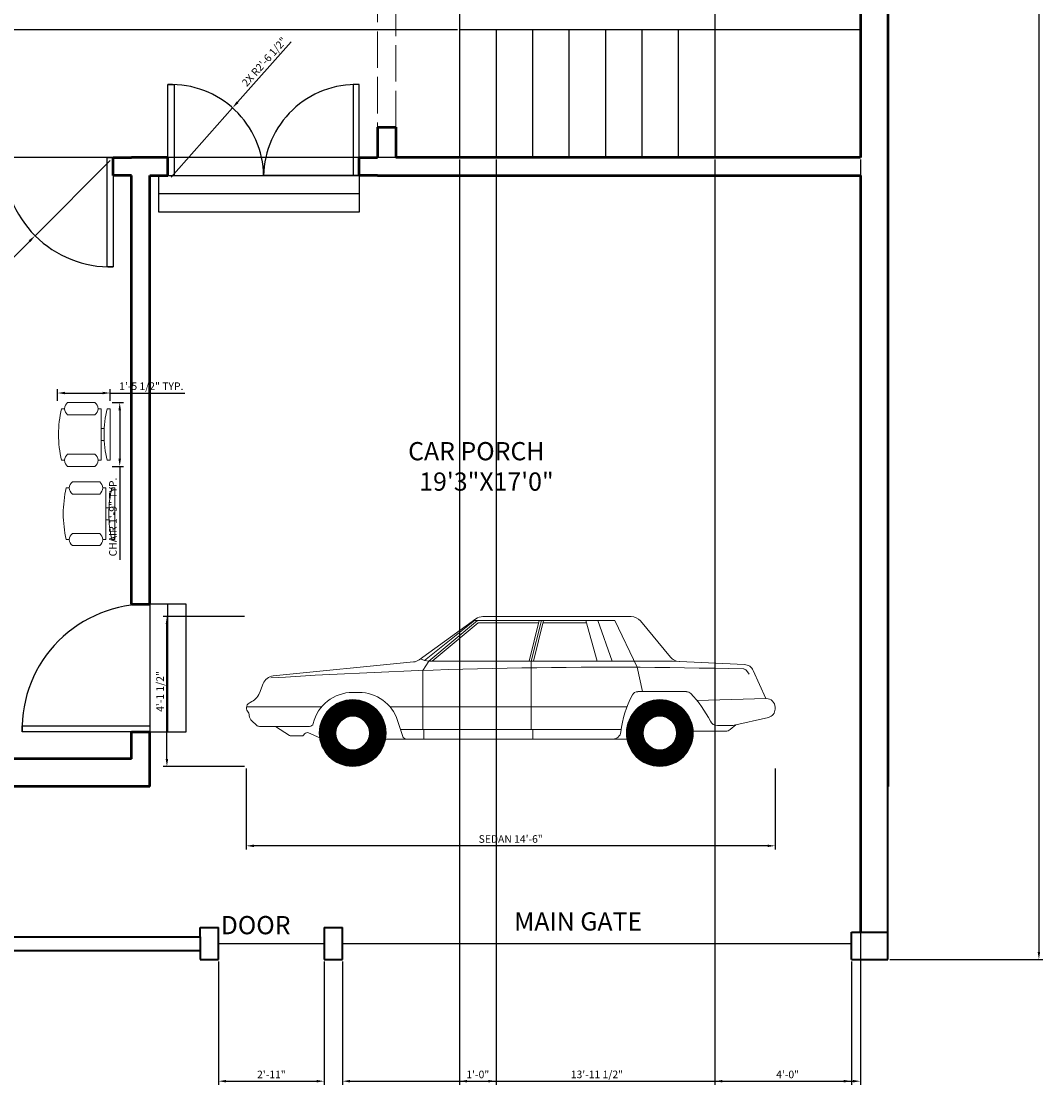
# Model space of a CAD drawing. Units: inches. Extents: x 2690 to 3266, y 1440 to 2261.
# Tile 2 of 4: x 2930 to 3266, y 1440 to 1790. Entities that reach past the tile are written whole.
import ezdxf

# ---------------------------------------------------------------- set-up
doc = ezdxf.new("R2010")
doc.units = ezdxf.units.IN
doc.linetypes.add('ACAD_ISO02W100', pattern=[15, 12, -3])
for name, color, linetype, lineweight in [('A-ANNO-DIMS', 2, 'Continuous', 18), ('A-ANNO-TEXT', 7, 'Continuous', 18), ('A-AREA-IDEN', 7, 'Continuous', 25), ('A-DOOR', 4, 'Continuous', 25), ('A-FLOR-STRS', 7, 'Continuous', 25), ('A-FURN', 8, 'Continuous', 18), ('A-SITE-VEHI', 9, 'Continuous', 13), ('A-WALL', 7, 'Continuous', 50), ('A-WALL-OVHD', 8, 'ACAD_ISO02W100', 18), ('L-SITE-GATE', 4, 'Continuous', 25), ('L-SITE-WALL', 7, 'Continuous', 35)]:
    doc.layers.add(name, color=color, linetype=linetype, lineweight=lineweight)
doc.styles.get("Standard").update_dxf_attribs({"font": 'arial.ttf'})
doc.dimstyles.new('ISO-25', dxfattribs={"dimtxt": 2.5, "dimasz": 2.5, "dimexe": 1.25, "dimexo": 0.625, "dimtad": 1, "dimlunit": 3, "dimtxsty": 'Standard', "dimcen": 2.5, "dimadec": 0, "dimazin": 0, "dimtfac": 1, "dimtmove": 0, "dimatfit": 3, "dimfxl": 1, "dimarcsym": 0})

# ---------------------------------------------------------------- blocks, each defined once
blk = doc.blocks.new('Chair - Desk')
for p, q in [((-8.5, 0), (-8.5, -1)), ((-8.5, 0), (8.5, 0)), ((8.5, 0), (8.5, -1)), ((-8.5, -3), (-8.5, -4)), ((-8.5, -3), (8.5, -3)), ((-2, -3), (-2, -1.9355)), ((2, -1.9576), (2, -3)), ((8.5, -3), (8.5, -4)), ((-10.5, -5), (-10.5, -14)), ((-6.5, -14), (-6.5, -5)), ((6.5, -5), (6.5, -14)), ((10.5, -14), (10.5, -5)), ((-8.5, -15), (-8.5, -16)), ((8.5, -15), (8.5, -16))]:
    blk.add_line(p, q)
for centre, radius, start, end in [((0, 34.625), 36.625, 256.5803, 283.4197), ((-8.5, -6.5), 2.5, 36.8699, 143.1301), ((8.5, -6.5), 2.5, 36.8699, 143.1301), ((-8.5, -12.5), 2.5, 216.8699, 323.1301), ((8.5, -12.5), 2.5, 216.8699, 323.1301), ((0, 19.625), 36.625, 256.5803, 283.4197)]:
    blk.add_arc(centre, radius, start, end)
blk = doc.blocks.new('Car - sedan  side')
for p, q in [((-77.81, 49.34), (-126.58, 49.34)), ((-139.53, 35.99), (-129.64, 47.91)), ((-128.57, 32.64), (-121.22, 48.02)), ((-74.7, 48.02), (-121.22, 48.02)), ((-120.32, 34.67), (-115.67, 48.02)), ((-115.4, 34.67), (-111.74, 48.02)), ((-97.55, 47.3), (-111.94, 47.3)), ((-94.41, 34.67), (-97.73, 48.02)), ((-93.72, 34.67), (-97.04, 48.02)), ((-93.03, 34.67), (-96.34, 48.02)), ((-76.26, 47.3), (-96.16, 47.3)), ((-61.08, 34.66), (-76.26, 47.3)), ((-60.02, 34.65), (-76.07, 48.02)), ((-56.87, 35.13), (-75.48, 48.59)), ((-58.54, 34.93), (-74.99, 48.02)), ((-57.21, 35.38), (-58.54, 34.93)), ((-164.57, 31.6), (-165.48, 30.35)), ((-140.23, 34.67), (-163.88, 33.56)), ((-62.28, 34.67), (-140.23, 34.67)), ((-130.39, 24.63), (-128.57, 32.64)), ((-93.72, 19.62), (-93.72, 34.67)), ((-62.28, 34.67), (-60.02, 34.65)), ((-60.02, 34.65), (-58.54, 34.93)), ((-57.97, 31.61), (-60.02, 34.65)), ((-57.97, 19.62), (-57.97, 31.61)), ((-54.93, 34.4), (-8.75, 29.8)), ((-170.93, 22.32), (-166.81, 31.56)), ((-128.78, 24.63), (-144.79, 24.63)), ((-4.21, 24.18), (-5.42, 27.27)), ((-148.26, 21.7), (-171.11, 22.33)), ((-36.97, 24.38), (-34.94, 24.38)), ((-174, 19.51), (-174, 18.91)), ((-47.2, 19.62), (-125.23, 19.62)), ((-93.72, 12.14), (-93.72, 19.62)), ((-57.97, 12.14), (-57.97, 19.62)), ((0, 19.62), (-24.7, 19.62)), ((-160.12, 13.48), (-171.81, 16.16)), ((-51.4, 9.89), (-49.69, 15.14)), ((-3.22, 13.59), (-1.77, 14.97)), ((-159.22, 12.14), (-161.08, 13.7)), ((-155.01, 13.48), (-160.12, 13.48)), ((-147.03, 11.6), (-157.73, 11.6)), ((-50.67, 12.14), (-123.32, 12.14)), ((-94.21, 9.03), (-94.21, 12.14)), ((-58.39, 9.03), (-58.39, 12.14)), ((-20.36, 11.06), (-24.06, 9.44)), ((-4.23, 13.19), (-20.72, 13.19)), ((-18.83, 10.42), (-19.11, 10.76)), ((-9.5, 13.19), (-14.1, 10.2)), ((-120.62, 9.03), (-125.23, 9.03)), ((-45.76, 9.03), (-120.62, 9.03)), ((-14.68, 10.03), (-18.01, 10.03))]:
    blk.add_line(p, q)
at = {"const_width": 5.49}
for points in [[(-127.8, 11, -1), (-144.3, 11, -1)], [(-26.69, 11, -1), (-43.19, 11, -1)]]:
    blk.add_lwpolyline(points, format="xyb", close=True, dxfattribs=at)
for centre, radius in [((-136.05, 11), 11), ((-34.94, 11), 11), ((-136.05, 11), 5.51), ((-34.94, 11), 5.51)]:
    blk.add_circle(centre, radius)
for centre, radius, start, end in [((-126.58, 45.38), 3.97, 90, 140.3029), ((-77.81, 45.38), 3.97, 54.135, 90), ((-142.58, 38.53), 3.97, 272.6827, 320.3029), ((-54.54, 38.35), 3.97, 234.135, 264.3123), ((-163.72, 30.18), 3.38, 92.6827, 155.9736), ((-163.62, 30.91), 1.17, 91.491, 143.9553), ((-118.51, -1702.12), 1734.79, 86.34698, 91.49105), ((-9.15, 25.82), 4, 21.3107, 84.3123), ((-144.79, 22.64), 1.98, 90, 136.3964), ((-128.78, 22.64), 1.98, 28.1371, 90), ((-171.18, 19.51), 2.82, 88.4193, 180), ((-118.09, -2.78), 38.85, 136.3964, 152.9097), ((-157.14, 7.48), 34.14, 6.5135, 28.1371), ((-36.97, 11), 13.38, 90, 161.9732), ((-34.94, 11), 13.38, 13.5864, 90), ((0.9, 26.18), 5.49, 201.3107, 247.7048), ((-1.92, 19.3), 1.94, 325.3744, 67.7048), ((-171.18, 18.91), 2.82, 180, 257.0905), ((2.46, 16.28), 3.37, 145.3744, 172.3839), ((-155.01, 16.1), 2.62, 270, 332.9097), ((-20.72, 14.43), 1.24, 193.5864, 270), ((-3.82, 17.12), 2.96, 313.7173, 352.3839), ((-157.73, 13.93), 2.32, 230.1291, 270), ((-120.62, 11.65), 2.62, 186.5135, 270), ((-19.93, 10.09), 1.06, 39.301, 113.7159), ((-4.23, 14.65), 1.46, 270, 313.7173), ((-52.58, 10.27), 1.24, 270, 341.9732), ((-18.01, 11.09), 1.06, 219.301, 270), ((-14.68, 11.09), 1.06, 270, 303.047)]:
    blk.add_arc(centre, radius, start, end)
blk = doc.blocks.new('*D15')
at = {"layer": 'A-ANNO-DIMS', "color": 0, "lineweight": -2, "transparency": 16777216}
for p, q in [((3216.1, 2204.49), (3266.46, 2204.49)), ((3265.21, 2201.99), (3265.21, 1483.99)), ((3216.1, 1481.49), (3266.46, 1481.49))]:
    blk.add_line(p, q, dxfattribs=at)
at = {"layer": 'A-ANNO-DIMS', "color": 0, "transparency": 16777216}
for points in [[(3264.79, 2201.99), (3265.63, 2201.99), (3265.21, 2204.49)], [(3264.79, 1483.99), (3265.63, 1483.99), (3265.21, 1481.49)]]:
    blk.add_solid(points, dxfattribs=at)
at = {"layer": 'Defpoints', "color": 0, "transparency": 16777216}
for p in [(3215.48, 2204.49), (3215.48, 1481.49), (3265.21, 1481.49)]:
    blk.add_point(p, dxfattribs=at)
at = {"layer": 'A-ANNO-DIMS', "color": 0, "transparency": 16777216, "insert": (3261.52, 1842.99), "char_height": 6, "attachment_point": 5, "rotation": 90}
blk.add_mtext('60\'-3"', dxfattribs=at)
blk = doc.blocks.new('DOOR-SWING-42IN')
for p, q in [((-42, 0), (-42, 2)), ((-42, 2), (0, 2)), ((0, 0), (-42, 0)), ((0, 2), (0, 0))]:
    blk.add_line(p, q)
blk.add_arc((-1, 1), 41.01, 88.6028, 181.3972)
blk = doc.blocks.new('*D21')
at = {"layer": 'A-ANNO-DIMS', "color": 0, "lineweight": -2, "transparency": 16777216}
for p, q in [((2960.07, 1664.79), (2963.85, 1664.79)), ((2962.6, 1662.29), (2962.6, 1646.29)), ((2960.07, 1643.79), (2963.85, 1643.79)), ((2962.6, 1643.79), (2962.6, 1613))]:
    blk.add_line(p, q, dxfattribs=at)
at = {"layer": 'A-ANNO-DIMS', "color": 0, "transparency": 16777216}
for points in [[(2962.18, 1662.29), (2963.01, 1662.29), (2962.6, 1664.79)], [(2962.18, 1646.29), (2963.01, 1646.29), (2962.6, 1643.79)]]:
    blk.add_solid(points, dxfattribs=at)
at = {"layer": 'Defpoints', "color": 0, "transparency": 16777216}
for p in [(2959.45, 1664.79), (2959.45, 1643.79), (2962.6, 1643.79)]:
    blk.add_point(p, dxfattribs=at)
at = {"layer": 'A-ANNO-DIMS', "color": 0, "transparency": 16777216, "insert": (2960.68, 1627.14), "char_height": 2.5, "attachment_point": 5, "rotation": 90}
blk.add_mtext('CHAIR 1\'-9" TYP.', dxfattribs=at)
blk = doc.blocks.new('*D22')
at = {"layer": 'A-ANNO-DIMS', "color": 0, "lineweight": -2, "transparency": 16777216}
for p, q in [((2942.11, 1665.42), (2942.11, 1669.19)), ((2959.45, 1665.42), (2959.45, 1669.19)), ((2944.61, 1667.94), (2956.95, 1667.94)), ((2959.45, 1667.94), (2984.03, 1667.94))]:
    blk.add_line(p, q, dxfattribs=at)
at = {"layer": 'A-ANNO-DIMS', "color": 0, "transparency": 16777216}
for points in [[(2944.61, 1668.36), (2944.61, 1667.53), (2942.11, 1667.94)], [(2956.95, 1668.36), (2956.95, 1667.53), (2959.45, 1667.94)]]:
    blk.add_solid(points, dxfattribs=at)
at = {"layer": 'Defpoints', "color": 0, "transparency": 16777216}
for p in [(2959.45, 1667.94), (2942.11, 1664.79), (2959.45, 1664.79)]:
    blk.add_point(p, dxfattribs=at)
at = {"layer": 'A-ANNO-DIMS', "color": 0, "transparency": 16777216, "insert": (2972.99, 1669.86), "char_height": 2.5, "attachment_point": 5}
blk.add_mtext('1\'-5 1/2" TYP.', dxfattribs=at)
blk = doc.blocks.new('*D47')
at = {"layer": 'A-ANNO-DIMS', "color": 0, "lineweight": -2, "transparency": 16777216}
for p, q in [((3004.25, 1544.4), (3004.25, 1517.66)), ((3178.36, 1544.4), (3178.36, 1517.66)), ((3175.86, 1518.91), (3006.75, 1518.91))]:
    blk.add_line(p, q, dxfattribs=at)
at = {"layer": 'A-ANNO-DIMS', "color": 0, "transparency": 16777216}
for points in [[(3006.75, 1519.32), (3006.75, 1518.49), (3004.25, 1518.91)], [(3175.86, 1519.32), (3175.86, 1518.49), (3178.36, 1518.91)]]:
    blk.add_solid(points, dxfattribs=at)
at = {"layer": 'Defpoints', "color": 0, "transparency": 16777216}
for p in [(3004.25, 1545.03), (3178.36, 1545.03), (3004.25, 1518.91)]:
    blk.add_point(p, dxfattribs=at)
at = {"layer": 'A-ANNO-DIMS', "color": 0, "transparency": 16777216, "insert": (3091.31, 1520.83), "char_height": 2.5, "attachment_point": 5}
blk.add_mtext('SEDAN 14\'-6"', dxfattribs=at)
blk = doc.blocks.new('*D48')
at = {"layer": 'A-ANNO-DIMS', "color": 0, "lineweight": -2, "transparency": 16777216}
for p, q in [((3003.62, 1594.37), (2976.88, 1594.37)), ((2978.13, 1547.53), (2978.13, 1591.87)), ((3003.62, 1545.03), (2976.88, 1545.03))]:
    blk.add_line(p, q, dxfattribs=at)
at = {"layer": 'A-ANNO-DIMS', "color": 0, "transparency": 16777216}
for points in [[(2977.72, 1591.87), (2978.55, 1591.87), (2978.13, 1594.37)], [(2977.72, 1547.53), (2978.55, 1547.53), (2978.13, 1545.03)]]:
    blk.add_solid(points, dxfattribs=at)
at = {"layer": 'Defpoints', "color": 0, "transparency": 16777216}
for p in [(2978.13, 1594.37), (3004.25, 1594.37), (3004.25, 1545.03)]:
    blk.add_point(p, dxfattribs=at)
at = {"layer": 'A-ANNO-DIMS', "color": 0, "transparency": 16777216, "insert": (2976.21, 1569.7), "char_height": 2.5, "attachment_point": 5, "rotation": 90}
blk.add_mtext('4\'-1 1/2"', dxfattribs=at)
blk = doc.blocks.new('*D49')
at = {"layer": 'A-ANNO-DIMS', "color": 0, "lineweight": -2, "transparency": 16777216}
for p, q in [((2995.13, 1480.86), (2995.13, 1440.19)), ((3029.93, 1480.86), (3029.93, 1440.19)), ((2997.63, 1441.44), (3027.43, 1441.44))]:
    blk.add_line(p, q, dxfattribs=at)
at = {"layer": 'A-ANNO-DIMS', "color": 0, "transparency": 16777216}
for points in [[(2997.63, 1441.85), (2997.63, 1441.02), (2995.13, 1441.44)], [(3027.43, 1441.85), (3027.43, 1441.02), (3029.93, 1441.44)]]:
    blk.add_solid(points, dxfattribs=at)
at = {"layer": 'Defpoints', "color": 0, "transparency": 16777216}
for p in [(2995.13, 1481.49), (3029.93, 1481.49), (3029.93, 1441.44)]:
    blk.add_point(p, dxfattribs=at)
at = {"layer": 'A-ANNO-DIMS', "color": 0, "transparency": 16777216, "insert": (3012.53, 1443.32), "char_height": 2.5, "attachment_point": 5}
blk.add_mtext('2\'-11"', dxfattribs=at)
blk = doc.blocks.new('*D50')
at = {"layer": 'A-ANNO-DIMS', "color": 0, "lineweight": -2, "transparency": 16777216}
for p, q in [((3035.93, 1480.86), (3035.93, 1440.19)), ((3203.48, 1480.86), (3203.48, 1440.19)), ((3038.43, 1441.44), (3200.98, 1441.44))]:
    blk.add_line(p, q, dxfattribs=at)
at = {"layer": 'A-ANNO-DIMS', "color": 0, "transparency": 16777216}
for points in [[(3038.43, 1441.85), (3038.43, 1441.02), (3035.93, 1441.44)], [(3200.98, 1441.85), (3200.98, 1441.02), (3203.48, 1441.44)]]:
    blk.add_solid(points, dxfattribs=at)
at = {"layer": 'Defpoints', "color": 0, "transparency": 16777216}
for p in [(3035.93, 1481.49), (3203.48, 1481.49), (3203.48, 1441.44)]:
    blk.add_point(p, dxfattribs=at)
at = {"layer": 'A-ANNO-DIMS', "color": 0, "transparency": 16777216, "insert": (3119.7, 1443.35), "char_height": 2.5, "attachment_point": 5}
blk.add_mtext('13\'-11 1/2"', dxfattribs=at)
blk = doc.blocks.new('*D51')
at = {"layer": 'A-ANNO-DIMS', "color": 0, "lineweight": -2, "transparency": 16777216}
for p, q in [((3074.48, 1744.86), (3074.48, 1440.19)), ((3086.48, 1744.86), (3086.48, 1440.19)), ((3076.98, 1441.44), (3083.98, 1441.44))]:
    blk.add_line(p, q, dxfattribs=at)
at = {"layer": 'A-ANNO-DIMS', "color": 0, "transparency": 16777216}
for points in [[(3076.98, 1441.85), (3076.98, 1441.02), (3074.48, 1441.44)], [(3083.98, 1441.85), (3083.98, 1441.02), (3086.48, 1441.44)]]:
    blk.add_solid(points, dxfattribs=at)
at = {"layer": 'Defpoints', "color": 0, "transparency": 16777216}
for p in [(3074.48, 1745.49), (3086.48, 1745.49), (3086.48, 1441.44)]:
    blk.add_point(p, dxfattribs=at)
at = {"layer": 'A-ANNO-DIMS', "color": 0, "transparency": 16777216, "insert": (3080.48, 1443.34), "char_height": 2.5, "attachment_point": 5}
blk.add_mtext('1\'-0"', dxfattribs=at)
blk = doc.blocks.new('*D52')
at = {"layer": 'A-ANNO-DIMS', "color": 0, "lineweight": -2, "transparency": 16777216}
for p, q in [((3158.48, 1744.86), (3158.48, 1440.19)), ((3206.48, 1744.86), (3206.48, 1440.19)), ((3160.98, 1441.44), (3203.98, 1441.44))]:
    blk.add_line(p, q, dxfattribs=at)
at = {"layer": 'A-ANNO-DIMS', "color": 0, "transparency": 16777216}
for points in [[(3160.98, 1441.85), (3160.98, 1441.02), (3158.48, 1441.44)], [(3203.98, 1441.85), (3203.98, 1441.02), (3206.48, 1441.44)]]:
    blk.add_solid(points, dxfattribs=at)
at = {"layer": 'Defpoints', "color": 0, "transparency": 16777216}
for p in [(3158.48, 1745.49), (3206.48, 1745.49), (3206.48, 1441.44)]:
    blk.add_point(p, dxfattribs=at)
at = {"layer": 'A-ANNO-DIMS', "color": 0, "transparency": 16777216, "insert": (3182.48, 1443.34), "char_height": 2.5, "attachment_point": 5}
blk.add_mtext('4\'-0"', dxfattribs=at)
blk = doc.blocks.new('*D53')
at = {"layer": 'A-ANNO-DIMS', "color": 0, "lineweight": -2, "transparency": 16777216}
for p, q in [((3073.85, 1787.49), (2694.18, 1787.49)), ((2695.43, 1747.99), (2695.43, 1784.99)), ((3073.85, 1745.49), (2694.18, 1745.49))]:
    blk.add_line(p, q, dxfattribs=at)
at = {"layer": 'A-ANNO-DIMS', "color": 0, "transparency": 16777216}
for points in [[(2695.01, 1784.99), (2695.84, 1784.99), (2695.43, 1787.49)], [(2695.01, 1747.99), (2695.84, 1747.99), (2695.43, 1745.49)]]:
    blk.add_solid(points, dxfattribs=at)
at = {"layer": 'Defpoints', "color": 0, "transparency": 16777216}
for p in [(2695.43, 1787.49), (3074.48, 1787.49), (3074.48, 1745.49)]:
    blk.add_point(p, dxfattribs=at)
at = {"layer": 'A-ANNO-DIMS', "color": 0, "transparency": 16777216, "insert": (2693.52, 1766.49), "char_height": 2.5, "attachment_point": 5, "rotation": 90}
blk.add_mtext('3\'-6"', dxfattribs=at)
blk = doc.blocks.new('*D60')
at = {"layer": 'A-ANNO-DIMS', "color": 0, "lineweight": -2, "transparency": 16777216}
for p, q in [((3019.04, 1783.53), (3001.4, 1763.67)), ((2979.48, 1739), (2999.74, 1761.8))]:
    blk.add_line(p, q, dxfattribs=at)
at = {"layer": 'A-ANNO-DIMS', "color": 0, "transparency": 16777216}
blk.add_solid([(3001.08, 1763.95), (3001.71, 1763.4), (2999.74, 1761.8)], dxfattribs=at)
at = {"layer": 'Defpoints', "color": 0, "transparency": 16777216}
for p in [(2999.74, 1761.8), (2979.48, 1739)]:
    blk.add_point(p, dxfattribs=at)
at = {"layer": 'A-ANNO-DIMS', "color": 0, "transparency": 16777216, "insert": (3010.46, 1776.76), "char_height": 2.5, "attachment_point": 5, "rotation": 48.3827}
blk.add_mtext('2X R2\'-6 1/2"', dxfattribs=at)
blk = doc.blocks.new('*D61')
at = {"layer": 'A-ANNO-DIMS', "color": 0, "lineweight": -2, "transparency": 16777216}
for p, q in [((2959.48, 1744.49), (2934.72, 1719.73)), ((2915.54, 1700.55), (2932.95, 1717.96))]:
    blk.add_line(p, q, dxfattribs=at)
at = {"layer": 'A-ANNO-DIMS', "color": 0, "transparency": 16777216}
blk.add_solid([(2932.65, 1718.25), (2933.24, 1717.66), (2934.72, 1719.73)], dxfattribs=at)
at = {"layer": 'Defpoints', "color": 0, "transparency": 16777216}
for p in [(2959.48, 1744.49), (2934.72, 1719.73)]:
    blk.add_point(p, dxfattribs=at)
at = {"layer": 'A-ANNO-DIMS', "color": 0, "transparency": 16777216, "insert": (2918.53, 1706.2), "char_height": 2.5, "attachment_point": 5, "rotation": 44.9992}
blk.add_mtext('R2\'-11"', dxfattribs=at)

msp = doc.modelspace()

# ---------------------------------------------------------------- linework, layer by layer
at = {"layer": 'A-DOOR'}
for p, q in [((2978.476, 1739.486), (2978.476, 1769.486)), ((2978.476, 1769.486), (2980.476, 1769.486)), ((2980.476, 1769.486), (2980.476, 1739.486)), ((3041.476, 1769.486), (3039.476, 1769.486)), ((3039.476, 1769.486), (3039.476, 1739.486)), ((3041.476, 1739.486), (3041.476, 1769.486)), ((2958.476, 1709.486), (2958.476, 1745.486)), ((2958.476, 1745.486), (2960.476, 1745.486)), ((2960.476, 1745.486), (2960.476, 1709.486)), ((2978.476, 1739.486), (3041.476, 1739.486)), ((3041.476, 1739.486), (3009.976, 1739.486)), ((3009.976, 1739.486), (3041.476, 1739.486)), ((2960.476, 1709.486), (2958.476, 1709.486))]:
    msp.add_line(p, q, dxfattribs=at)
for centre, radius, start, end in [((2979.476, 1738.998), 30.504, 0.91572, 91.87865), ((3040.476, 1738.998), 30.504, 88.12135, 179.08428), ((2959.476, 1744.486), 35.014, 178.36342, 271.63658)]:
    msp.add_arc(centre, radius, start, end, dxfattribs=at)
at = {"layer": 'A-FLOR-STRS'}
for p, q in [((3158.476, 1839.486), (3158.476, 1745.486)), ((3074.476, 1797.486), (3074.476, 1745.486)), ((3206.476, 1787.486), (3074.476, 1787.486)), ((3086.476, 1787.486), (3086.476, 1745.486)), ((3098.476, 1787.486), (3098.476, 1745.486)), ((3110.476, 1787.486), (3110.476, 1745.486)), ((3122.476, 1787.486), (3122.476, 1745.486)), ((3134.476, 1787.486), (3134.476, 1745.486)), ((3146.476, 1787.486), (3146.476, 1745.486)), ((2975.476, 1727.486), (2975.476, 1739.486)), ((3041.476, 1739.486), (3041.476, 1727.486)), ((3041.476, 1733.486), (2975.476, 1733.486)), ((3041.476, 1727.486), (2975.476, 1727.486)), ((2984.476, 1598.397), (2972.476, 1598.397)), ((2972.476, 1598.397), (2972.476, 1556.397)), ((2978.476, 1556.397), (2978.476, 1598.397)), ((2984.476, 1556.397), (2984.476, 1598.397)), ((2972.476, 1556.397), (2984.476, 1556.397)), ((2972.476, 1556.397), (2978.476, 1556.397))]:
    msp.add_line(p, q, dxfattribs=at)
at = {"layer": 'A-WALL'}
for p, q in [((3215.476, 2204.486), (3215.476, 1538.486)), ((3206.476, 1839.486), (3206.476, 1745.486)), ((3047.476, 1755.439), (3047.476, 1745.486)), ((3047.476, 1755.439), (3053.476, 1755.439)), ((3053.476, 1755.439), (3053.476, 1745.486)), ((2960.476, 1739.486), (2960.476, 1745.486)), ((2960.476, 1745.486), (2966.476, 1745.486)), ((2978.476, 1745.486), (2966.476, 1745.486)), ((2978.476, 1739.486), (2978.476, 1745.486)), ((3041.476, 1739.486), (3041.476, 1745.486)), ((3041.476, 1745.486), (3047.476, 1745.486)), ((3206.476, 1745.486), (3053.476, 1745.486)), ((2966.476, 1739.486), (2960.476, 1739.486)), ((2966.476, 1598.397), (2966.476, 1739.486)), ((2972.476, 1739.486), (2978.476, 1739.486)), ((2972.476, 1739.486), (2978.476, 1739.486)), ((2972.476, 1598.397), (2972.476, 1739.486)), ((3047.476, 1739.486), (3041.476, 1739.486)), ((3047.476, 1739.486), (3206.476, 1739.486)), ((3206.476, 1739.486), (3206.476, 1490.486)), ((2966.476, 1598.397), (2972.476, 1598.397)), ((2966.476, 1547.486), (2966.476, 1556.397)), ((2966.476, 1556.397), (2972.476, 1556.397)), ((2972.476, 1538.486), (2972.476, 1556.397)), ((2966.476, 1547.486), (2744.476, 1547.486)), ((2972.476, 1538.486), (2735.476, 1538.486))]:
    msp.add_line(p, q, dxfattribs=at)
at = {"layer": 'A-WALL-OVHD'}
for p, q in [((3047.476, 1831.977), (3047.476, 1755.439)), ((3053.476, 1755.439), (3053.476, 1831.977))]:
    msp.add_line(p, q, dxfattribs=at)
at = {"layer": 'L-SITE-GATE'}
for p, q in [((2995.13, 1486.736), (3029.933, 1486.736)), ((3035.933, 1486.736), (3203.476, 1486.736))]:
    msp.add_line(p, q, dxfattribs=at)
at = {"layer": 'L-SITE-WALL'}
for p, q in [((3206.476, 1490.486), (3206.476, 1538.486)), ((3215.476, 1484.486), (3215.476, 1538.486)), ((2989.13, 1488.986), (2989.13, 1491.986)), ((2989.13, 1491.986), (2995.13, 1491.986)), ((2995.13, 1481.486), (2995.13, 1491.986)), ((3029.933, 1491.986), (3035.933, 1491.986)), ((3029.933, 1491.986), (3029.933, 1481.486)), ((3035.933, 1481.486), (3035.933, 1491.986)), ((3203.476, 1481.486), (3203.476, 1490.486)), ((3203.476, 1490.486), (3215.476, 1490.486)), ((2739.976, 1488.986), (2989.13, 1488.986)), ((2989.13, 1488.986), (2989.13, 1481.486)), ((2735.476, 1484.486), (2989.13, 1484.486)), ((3215.476, 1481.486), (3215.476, 1484.486)), ((2989.13, 1481.486), (2995.13, 1481.486)), ((3029.933, 1481.486), (3035.933, 1481.486)), ((3203.476, 1481.486), (3215.476, 1481.486))]:
    msp.add_line(p, q, dxfattribs=at)

# ---------------------------------------------------------------- block references
at = {"layer": 'A-DOOR'}
msp.add_blockref('DOOR-SWING-42IN', (2972.476, 1556.397), dxfattribs=at)
at = {"layer": 'A-FURN', "rotation": 270}
for p in [(2959.447, 1654.292), (2961.003, 1628.205)]:
    msp.add_blockref('Chair - Desk', p, dxfattribs=at)
at = {"layer": 'A-SITE-VEHI', "xscale": -1}
msp.add_blockref('Car - sedan  side', (3004.363, 1545.025), dxfattribs=at)

# ---------------------------------------------------------------- texts
at = {"layer": 'A-ANNO-TEXT', "char_height": 6, "attachment_point": 1}
for s, insert in [(' DOOR', (2994.009, 1495.801)), (' MAIN GATE', (3090.623, 1497.025))]:
    msp.add_mtext_dynamic_manual_height_columns(s, width=77.52183, gutter_width=12.5, heights=[0], dxfattribs=dict(at, insert=insert))
at = {"layer": 'A-AREA-IDEN', "insert": (3055.716, 1651.802), "char_height": 6, "attachment_point": 1}
msp.add_mtext_dynamic_manual_height_columns(' CAR PORCH\\P   19\'3"X17\'0"', width=77.52183, gutter_width=12.5, heights=[0], dxfattribs=at)

# ---------------------------------------------------------------- dimensions: what is measured, and where the dimension line sits
at = {"layer": 'A-ANNO-DIMS'}
for base, p1, p2, override, picture, middle in [((3265.21, 1481.486), (3215.476, 2204.486), (3215.476, 1481.486), {"dimtxt": 6, "dimclrd": 0, "dimclre": 0, "dimclrt": 0}, '*D15', (3261.519, 1842.986)), ((2695.426, 1787.486), (3074.476, 1745.486), (3074.476, 1787.486), {"dimdec": 1, "dimlfac": 1, "dimrnd": 0, "dimzin": 1, "dimdsep": 46, "dimlunit": 4, "dimfrac": 2}, '*D53', (2693.524, 1766.486)), ((2978.133, 1594.37), (3004.25, 1545.025), (3004.25, 1594.37), {"dimdec": 1, "dimlfac": 1, "dimrnd": 0, "dimzin": 1, "dimdsep": 46, "dimlunit": 4, "dimfrac": 2}, '*D48', (2976.215, 1569.698))]:
    dim = msp.add_linear_dim(base=base, p1=p1, p2=p2, angle=90, dimstyle='ISO-25', override=override, dxfattribs=at)
    dim.commit()
    dim.dimension.update_dxf_attribs({"geometry": picture, "text_midpoint": middle})
dim = msp.add_radius_dim(center=(2979.476, 1738.998), mpoint=(2999.736, 1761.803), text='2X <>', dimstyle='ISO-25', override={"dimdec": 1, "dimlfac": 1, "dimrnd": 0, "dimzin": 1, "dimdsep": 46, "dimlunit": 4, "dimfrac": 2}, dxfattribs=at)
dim.commit()
dim.dimension.update_dxf_attribs({"geometry": '*D60', "text_midpoint": (3011.891, 1775.486), "dimtype": 164})
dim = msp.add_radius_dim(center=(2959.476, 1744.486), mpoint=(2934.717, 1719.727), dimstyle='ISO-25', override={"dimdec": 1, "dimlfac": 1, "dimrnd": 0, "dimzin": 1, "dimdsep": 46, "dimlunit": 4, "dimfrac": 2}, dxfattribs=at)
dim.commit()
dim.dimension.update_dxf_attribs({"geometry": '*D61', "text_midpoint": (2919.862, 1704.872), "dimtype": 164})
for base, p1, p2, picture, middle in [((3086.476, 1441.436), (3074.476, 1745.486), (3086.476, 1745.486), '*D51', (3080.476, 1443.337)), ((3206.476, 1441.436), (3158.476, 1745.486), (3206.476, 1745.486), '*D52', (3182.476, 1443.337)), ((3029.933, 1441.436), (2995.13, 1481.486), (3029.933, 1481.486), '*D49', (3012.531, 1443.316)), ((3203.476, 1441.436), (3035.933, 1481.486), (3203.476, 1481.486), '*D50', (3119.705, 1443.354))]:
    dim = msp.add_linear_dim(base=base, p1=p1, p2=p2, dimstyle='ISO-25', override={"dimdec": 1, "dimlfac": 1, "dimrnd": 0, "dimzin": 1, "dimdsep": 46, "dimlunit": 4, "dimfrac": 2}, dxfattribs=at)
    dim.commit()
    dim.dimension.update_dxf_attribs({"geometry": picture, "text_midpoint": middle})
dim = msp.add_linear_dim(base=(2959.447, 1667.942), p1=(2942.113, 1664.792), p2=(2959.447, 1664.792), text='<> TYP.', dimstyle='ISO-25', override={"dimdec": 1, "dimlfac": 1, "dimrnd": 0, "dimzin": 1, "dimdsep": 46, "dimlunit": 4, "dimfrac": 2}, dxfattribs=at)
dim.commit()
dim.dimension.update_dxf_attribs({"geometry": '*D22', "text_midpoint": (2972.986, 1669.86)})
for base, p1, p2, angle, text, picture, middle in [((2962.597, 1643.792), (2959.447, 1664.792), (2959.447, 1643.792), 270, 'CHAIR <> TYP.', '*D21', (2960.679, 1627.144)), ((3004.25, 1518.908), (3178.363, 1545.025), (3004.25, 1545.025), 180, 'SEDAN <>', '*D47', (3091.306, 1520.826))]:
    dim = msp.add_linear_dim(base=base, p1=p1, p2=p2, angle=angle, text=text, dimstyle='ISO-25', override={"dimdec": 1, "dimlfac": 1, "dimrnd": 0, "dimzin": 1, "dimdsep": 46, "dimlunit": 4, "dimfrac": 2}, dxfattribs=at)
    dim.commit()
    dim.dimension.update_dxf_attribs({"geometry": picture, "text_midpoint": middle})

doc.saveas('drawing.dxf')
